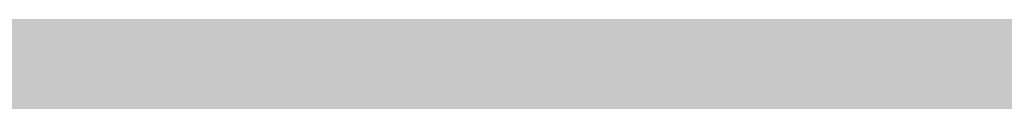
# Model space of a CAD drawing. Units: millimetres. Extents: x 0 to 2267, y 0 to 1823.
# Tile 51 of 256: x 1596.855 to 1600.369, y 1226.115 to 1226.386. Entities that reach past the tile are written whole.
import ezdxf

# ---------------------------------------------------------------- set-up
doc = ezdxf.new("R2010")
doc.units = ezdxf.units.MM
doc.header["$MEASUREMENT"] = 0
doc.layers.add('M-HATC', color=252, linetype='Continuous', lineweight=18)

msp = doc.modelspace()

# ---------------------------------------------------------------- hatches: boundary and pattern name
at = {"layer": 'M-HATC'}
h = msp.add_hatch(color=256, dxfattribs=at)
h.dxf.hatch_style = 1
h.paths.add_polyline_path([(2055.771, 1603.062), (1381.0868, 1603.062), (1381.0868, 1598.062), (2055.771, 1598.062)])
h.paths.add_polyline_path([(2055.771, 1598.062), (1381.0868, 1598.062), (1381.0868, 1593.062), (2055.771, 1593.062)])
h.paths.add_polyline_path([(2051.3074, 1536.7609), (1385.5504, 1536.7609), (1385.5504, 1526.7609), (1387.5504, 1526.7609), (1388.5366, 1525.0528), (1385.3319, 1521.2335), (1385.3319, 1521.2226), (2050.2542, 1522.7491), (2048.3212, 1525.0528), (2049.3074, 1526.7609), (2051.3074, 1526.7609)])
edge = h.paths.add_edge_path()
edge.add_arc((1847.5345, 1379.1492), 135, 222.603061, 222.890851, ccw=False)
edge.add_line((1748.1663, 1287.7656), (1683.0921, 1287.7656))
edge.add_arc((1583.7239, 1379.1492), 135, 317.109149, 317.396939, ccw=False)
edge.add_arc((1678.9686, 1290.6707), 5, 222.8909, 317.1091, ccw=False)
edge.add_arc((1774.2133, 1379.1492), 135, 222.603061, 222.890851, ccw=False)
edge.add_line((1674.8451, 1287.7656), (1609.7709, 1287.7656))
edge.add_arc((1510.4027, 1379.1492), 135, 317.109149, 317.396939, ccw=False)
edge.add_arc((1605.6474, 1290.6707), 5, 222.8909, 317.1091, ccw=False)
edge.add_arc((1700.8921, 1379.1492), 135, 222.603061, 222.890851, ccw=False)
edge.add_line((1601.5239, 1287.7656), (1536.4497, 1287.7656))
edge.add_arc((1437.0815, 1379.1492), 135, 317.109149, 317.396939, ccw=False)
edge.add_arc((1532.3262, 1290.6707), 5, 222.8909, 317.1091, ccw=False)
edge.add_arc((1627.5709, 1379.1492), 135, 222.603061, 222.890851, ccw=False)
edge.add_line((1528.2027, 1287.7656), (1505.9289, 1287.7656))
edge.add_spline(control_points=[(1505.9289, 1287.7656), (1504.2622, 1287.7656), (1504.2622, 1282.7656), (1505.9289, 1282.7656)], knot_values=[0, 0, 0, 0, 5, 5, 5, 5], degree=3, periodic=0)
edge.add_line((1505.9289, 1282.7656), (1930.9289, 1282.7656))
edge.add_spline(control_points=[(1930.9289, 1282.7656), (1932.5956, 1282.7656), (1932.5956, 1287.7656), (1930.9289, 1287.7656)], knot_values=[0, 0, 0, 0, 5, 5, 5, 5], degree=3, periodic=0)
edge.add_line((1930.9289, 1287.7656), (1903.0557, 1287.7656))
edge.add_arc((1803.6875, 1379.1492), 135, 317.109149, 317.396939, ccw=False)
edge.add_arc((1898.9322, 1290.6707), 5, 222.8909, 317.1091, ccw=False)
edge.add_arc((1994.1769, 1379.1492), 135, 222.603061, 222.890851, ccw=False)
edge.add_line((1894.8087, 1287.7656), (1829.7345, 1287.7656))
edge.add_arc((1730.3663, 1379.1492), 135, 317.109149, 317.396939, ccw=False)
edge.add_arc((1825.611, 1290.6707), 5, 222.8909, 317.1091, ccw=False)
edge.add_arc((1920.8557, 1379.1492), 135, 222.603061, 222.890851, ccw=False)
edge.add_line((1821.4875, 1287.7656), (1756.4133, 1287.7656))
edge.add_arc((1657.0451, 1379.1492), 135, 317.109149, 317.396939, ccw=False)
edge.add_arc((1752.2898, 1290.6707), 5, 222.8909, 317.1091, ccw=False)
edge = h.paths.add_edge_path()
edge.add_spline(control_points=[(1843.4289, 1227.2475), (1845.0956, 1227.2475), (1845.0956, 1232.2475), (1843.4289, 1232.2475)], knot_values=[0, 0, 0, 0, 5, 5, 5, 5], degree=3, periodic=0)
edge.add_line((1843.4289, 1232.2475), (1593.4289, 1232.2475))
edge.add_spline(control_points=[(1593.4289, 1232.2475), (1591.7622, 1232.2475), (1591.7622, 1227.2475), (1593.4289, 1227.2475)], knot_values=[0, 0, 0, 0, 5, 5, 5, 5], degree=3, periodic=0)
edge.add_line((1593.4289, 1227.2475), (1843.4289, 1227.2475))
h.paths.add_polyline_path([(1905.9289, 1127.4171), (1530.9289, 1127.4171, 0.414214), (1520.9289, 1117.4171), (1530.9289, 1117.4171), (1915.9289, 1117.4171, 0.414214)])
edge = h.paths.add_edge_path()
edge.add_arc((1397.0858, 1498.4078), 12.7299, 90.78215, 190.87871, ccw=False)
edge.add_line((1396.912, 1511.1365), (1428.0097, 1511.3488))
edge.add_line((1428.0097, 1511.3488), (1433.0097, 1511.3488))
edge.add_line((1433.0097, 1511.3488), (1434.439, 1511.3488))
edge.add_arc((1419.474, 1498.0804), 20, 41.561, 74.08211)
edge.add_line((1424.9592, 1517.3135), (1399.9351, 1517.2561))
edge.add_spline(control_points=[(1399.9307, 1517.2561), (1399.884, 1517.2131), (1399.8328, 1517.1689), (1399.7774, 1517.1236)], knot_values=[11.567499, 11.567499, 11.567499, 11.567499, 11.814249, 11.814249, 11.814249, 11.814249], degree=3, periodic=0)
edge.add_spline(control_points=[(1399.6328, 1517.0099), (1399.5831, 1516.9721), (1399.5307, 1516.9338), (1399.4759, 1516.8947)], knot_values=[11.167718, 11.167718, 11.167718, 11.167718, 11.365188, 11.365188, 11.365188, 11.365188], degree=3, periodic=0)
edge.add_spline(control_points=[(1399.3398, 1516.8001), (1399.1514, 1516.6719), (1398.9384, 1516.5377), (1398.704, 1516.3994)], knot_values=[10.376405, 10.376405, 10.376405, 10.376405, 11.00994, 11.00994, 11.00994, 11.00994], degree=3, periodic=0)
edge.add_spline(control_points=[(1398.6572, 1516.3719), (1398.5789, 1516.326), (1398.4983, 1516.2797), (1398.4155, 1516.2331)], knot_values=[10.125175, 10.125175, 10.125175, 10.125175, 10.334406, 10.334406, 10.334406, 10.334406], degree=3, periodic=0)
edge.add_spline(control_points=[(1398.2642, 1516.1487), (1398.196, 1516.1111), (1398.1263, 1516.0732), (1398.0555, 1516.0351)], knot_values=[9.832246, 9.832246, 9.832246, 9.832246, 9.999658, 9.999658, 9.999658, 9.999658], degree=3, periodic=0)
edge.add_spline(control_points=[(1397.9987, 1516.0048), (1397.7312, 1515.8621), (1397.446, 1515.7171), (1397.1466, 1515.5714)], knot_values=[9.161808, 9.161808, 9.161808, 9.161808, 9.787769, 9.787769, 9.787769, 9.787769], degree=3, periodic=0)
edge.add_spline(control_points=[(1397.1466, 1515.5714), (1396.8418, 1515.423), (1396.5222, 1515.274), (1396.1914, 1515.1262)], knot_values=[8.524455, 8.524455, 8.524455, 8.524455, 9.161808, 9.161808, 9.161808, 9.161808], degree=3, periodic=0)
edge.add_spline(control_points=[(1396.0777, 1515.0756), (1395.9854, 1515.0348), (1395.8922, 1514.994), (1395.7983, 1514.9534)], knot_values=[8.275193, 8.275193, 8.275193, 8.275193, 8.451726, 8.451726, 8.451726, 8.451726], degree=3, periodic=0)
edge.add_spline(control_points=[(1395.6018, 1514.8691), (1395.4997, 1514.8257), (1395.3968, 1514.7824), (1395.2932, 1514.7394)], knot_values=[7.962917, 7.962917, 7.962917, 7.962917, 8.152764, 8.152764, 8.152764, 8.152764], degree=3, periodic=0)
edge.add_spline(control_points=[(1395.2116, 1514.7057), (1394.8278, 1514.5475), (1394.4345, 1514.3929), (1394.0364, 1514.2442)], knot_values=[7.21254, 7.21254, 7.21254, 7.21254, 7.913148, 7.913148, 7.913148, 7.913148], degree=3, periodic=0)
edge.add_spline(control_points=[(1394.0364, 1514.2442), (1393.7076, 1514.1214), (1393.3754, 1514.0027), (1393.0427, 1513.8895)], knot_values=[6.633733, 6.633733, 6.633733, 6.633733, 7.21254, 7.21254, 7.21254, 7.21254], degree=3, periodic=0)
edge.add_spline(control_points=[(1392.8214, 1513.815), (1392.7198, 1513.7812), (1392.6181, 1513.7479), (1392.5166, 1513.7152)], knot_values=[6.328796, 6.328796, 6.328796, 6.328796, 6.505493, 6.505493, 6.505493, 6.505493], degree=3, periodic=0)
edge.add_spline(control_points=[(1392.5166, 1513.7152), (1392.3187, 1513.6515), (1392.1212, 1513.59), (1391.9244, 1513.531)], knot_values=[5.984605, 5.984605, 5.984605, 5.984605, 6.328796, 6.328796, 6.328796, 6.328796], degree=3, periodic=0)
edge.add_spline(control_points=[(1391.7915, 1513.4915), (1391.3122, 1513.3501), (1390.8384, 1513.2239), (1390.3784, 1513.1171)], knot_values=[5.066697, 5.066697, 5.066697, 5.066697, 5.907055, 5.907055, 5.907055, 5.907055], degree=3, periodic=0)
edge.add_spline(control_points=[(1390.3784, 1513.1171), (1390.1797, 1513.071), (1389.9836, 1513.0284), (1389.7907, 1512.9899)], knot_values=[4.70367, 4.70367, 4.70367, 4.70367, 5.066695, 5.066695, 5.066695, 5.066695], degree=3, periodic=0)
edge.add_spline(control_points=[(1389.422, 1512.9204), (1389.2459, 1512.8892), (1389.0729, 1512.8617), (1388.9036, 1512.8381)], knot_values=[4.130571, 4.130571, 4.130571, 4.130571, 4.469816, 4.469816, 4.469816, 4.469816], degree=3, periodic=0)
edge.add_spline(control_points=[(1388.9036, 1512.8381), (1388.591, 1512.7946), (1388.2911, 1512.7644), (1388.0071, 1512.7494)], knot_values=[3.504031, 3.504031, 3.504031, 3.504031, 4.130571, 4.130571, 4.130571, 4.130571], degree=3, periodic=0)
edge.add_spline(control_points=[(1387.9356, 1512.7459), (1387.8538, 1512.7423), (1387.7733, 1512.74), (1387.6944, 1512.739)], knot_values=[3.268866, 3.268866, 3.268866, 3.268866, 3.451164, 3.451164, 3.451164, 3.451164], degree=3, periodic=0)
edge.add_spline(control_points=[(1387.3351, 1512.7443), (1387.2076, 1512.7499), (1387.0847, 1512.7597), (1386.967, 1512.7739)], knot_values=[2.670686, 2.670686, 2.670686, 2.670686, 2.984, 2.984, 2.984, 2.984], degree=3, periodic=0)
edge.add_spline(control_points=[(1386.8327, 1512.7922), (1386.8209, 1512.7941), (1386.8092, 1512.7959), (1386.7975, 1512.7979)], knot_values=[2.516981, 2.516981, 2.516981, 2.516981, 2.549528, 2.549528, 2.549528, 2.549528], degree=3, periodic=0)
edge.add_spline(control_points=[(1386.4526, 1512.8735), (1386.4257, 1512.881), (1386.3993, 1512.889), (1386.3733, 1512.8972)], knot_values=[2.095869, 2.095869, 2.095869, 2.095869, 2.17941, 2.17941, 2.17941, 2.17941], degree=3, periodic=0)
edge.add_spline(control_points=[(1386.0691, 1513.0189), (1386.0634, 1513.0217), (1386.0577, 1513.0246), (1386.052, 1513.0275)], knot_values=[1.72453, 1.72453, 1.72453, 1.72453, 1.745933, 1.745933, 1.745933, 1.745933], degree=3, periodic=0)
edge.add_arc((1399.474, 1498.0804), 20, 131.82432, 180)
edge.add_arc((1630.3336, 1505.5484), 250.9708, 181.705176, 236.427975)
edge.add_arc((1605.3399, 1483.3044), 218.7822, 238.660829, 243.34961)
edge.add_arc((1647.0911, 1510.3592), 262.8986, 183.129836, 237.853442, ccw=False)
h.paths.add_polyline_path([(1406.5369, 1391.9644, 0.149382), (1491.5506, 1296.4418, -0.129517)], flags=17)
edge = h.paths.add_edge_path()
edge.add_arc((2037.3838, 1498.0804), 20, 0, 48.26587)
edge.add_spline(control_points=[(2050.6973, 1513.0052), (2050.6512, 1512.9847), (2050.6034, 1512.9655), (2050.5539, 1512.9477)], knot_values=[1.835652, 1.835652, 1.835652, 1.835652, 2.000781, 2.000781, 2.000781, 2.000781], degree=3, periodic=0)
edge.add_spline(control_points=[(2050.4616, 1512.9166), (2050.479, 1512.9221), (2050.4963, 1512.9277), (2050.5133, 1512.9335)], knot_values=[2.045477, 2.045477, 2.045477, 2.045477, 2.101389, 2.101389, 2.101389, 2.101389], degree=3, periodic=0)
edge.add_spline(control_points=[(2050.129, 1512.8342), (2050.1984, 1512.8473), (2050.2657, 1512.8623), (2050.3308, 1512.8792)], knot_values=[2.237629, 2.237629, 2.237629, 2.237629, 2.435841, 2.435841, 2.435841, 2.435841], degree=3, periodic=0)
edge.add_spline(control_points=[(2050.0946, 1512.8278), (2050.1061, 1512.8299), (2050.1176, 1512.832), (2050.129, 1512.8342)], knot_values=[2.435841, 2.435841, 2.435841, 2.435841, 2.468321, 2.468321, 2.468321, 2.468321], degree=3, periodic=0)
edge.add_spline(control_points=[(2049.7843, 1512.7851), (2049.8552, 1512.7922), (2049.9243, 1512.8008), (2049.9917, 1512.8109)], knot_values=[2.563852, 2.563852, 2.563852, 2.563852, 2.748541, 2.748541, 2.748541, 2.748541], degree=3, periodic=0)
edge.add_spline(control_points=[(2049.4052, 1512.7617), (2049.5364, 1512.7653), (2049.6629, 1512.773), (2049.7843, 1512.7851)], knot_values=[2.748541, 2.748541, 2.748541, 2.748541, 3.064882, 3.064882, 3.064882, 3.064882], degree=3, periodic=0)
edge.add_spline(control_points=[(2049.1698, 1512.7597), (2049.2336, 1512.7591), (2049.2965, 1512.7594), (2049.3584, 1512.7606)], knot_values=[3.102309, 3.102309, 3.102309, 3.102309, 3.2503, 3.2503, 3.2503, 3.2503], degree=3, periodic=0)
edge.add_spline(control_points=[(2048.8573, 1512.7691), (2048.9638, 1512.7638), (2049.068, 1512.7606), (2049.1698, 1512.7597)], knot_values=[3.2503, 3.2503, 3.2503, 3.2503, 3.486069, 3.486069, 3.486069, 3.486069], degree=3, periodic=0)
edge.add_spline(control_points=[(2048.6924, 1512.7789), (2048.3729, 1512.8009), (2048.0345, 1512.8411), (2047.6817, 1512.897)], knot_values=[3.606429, 3.606429, 3.606429, 3.606429, 4.2989, 4.2989, 4.2989, 4.2989], degree=3, periodic=0)
edge.add_spline(control_points=[(2047.6817, 1512.897), (2047.5458, 1512.9185), (2047.4077, 1512.9424), (2047.2678, 1512.9685)], knot_values=[4.2989, 4.2989, 4.2989, 4.2989, 4.565769, 4.565769, 4.565769, 4.565769], degree=3, periodic=0)
edge.add_spline(control_points=[(2047.2678, 1512.9685), (2047.1449, 1512.9914), (2047.0207, 1513.016), (2046.8951, 1513.0422)], knot_values=[4.565769, 4.565769, 4.565769, 4.565769, 4.799971, 4.799971, 4.799971, 4.799971], degree=3, periodic=0)
edge.add_spline(control_points=[(2046.8951, 1513.0422), (2046.5286, 1513.1188), (2046.1513, 1513.209), (2045.7676, 1513.3107)], knot_values=[4.799971, 4.799971, 4.799971, 4.799971, 5.483718, 5.483718, 5.483718, 5.483718], degree=3, periodic=0)
edge.add_spline(control_points=[(2045.7676, 1513.3107), (2045.3724, 1513.4154), (2044.9704, 1513.5322), (2044.5662, 1513.6588)], knot_values=[5.483718, 5.483718, 5.483718, 5.483718, 6.187866, 6.187866, 6.187866, 6.187866], degree=3, periodic=0)
edge.add_spline(control_points=[(2044.5662, 1513.6588), (2044.4149, 1513.7061), (2044.2633, 1513.7549), (2044.1116, 1513.8048)], knot_values=[6.187866, 6.187866, 6.187866, 6.187866, 6.451551, 6.451551, 6.451551, 6.451551], degree=3, periodic=0)
edge.add_spline(control_points=[(2044.1116, 1513.8048), (2043.9967, 1513.8427), (2043.8817, 1513.8813), (2043.7668, 1513.9205)], knot_values=[6.451551, 6.451551, 6.451551, 6.451551, 6.651434, 6.651434, 6.651434, 6.651434], degree=3, periodic=0)
edge.add_spline(control_points=[(2043.7668, 1513.9205), (2043.3716, 1514.0554), (2042.9774, 1514.1979), (2042.5886, 1514.3458)], knot_values=[6.651434, 6.651434, 6.651434, 6.651434, 7.338879, 7.338879, 7.338879, 7.338879], degree=3, periodic=0)
edge.add_spline(control_points=[(2042.5886, 1514.3458), (2042.1643, 1514.5071), (2041.7465, 1514.6749), (2041.3409, 1514.846)], knot_values=[7.338879, 7.338879, 7.338879, 7.338879, 8.089209, 8.089209, 8.089209, 8.089209], degree=3, periodic=0)
edge.add_spline(control_points=[(2041.3409, 1514.846), (2041.1028, 1514.9465), (2040.869, 1515.0481), (2040.6405, 1515.1502)], knot_values=[8.089209, 8.089209, 8.089209, 8.089209, 8.529587, 8.529587, 8.529587, 8.529587], degree=3, periodic=0)
edge.add_spline(control_points=[(2040.51, 1515.2089), (2040.0824, 1515.4022), (2039.6747, 1515.5971), (2039.295, 1515.7894)], knot_values=[8.613818, 8.613818, 8.613818, 8.613818, 9.44571, 9.44571, 9.44571, 9.44571], degree=3, periodic=0)
edge.add_spline(control_points=[(2039.295, 1515.7894), (2039.0618, 1515.9075), (2038.8391, 1516.0246), (2038.6288, 1516.1398)], knot_values=[9.44571, 9.44571, 9.44571, 9.44571, 9.956404, 9.956404, 9.956404, 9.956404], degree=3, periodic=0)
edge.add_spline(control_points=[(2038.6288, 1516.1398), (2038.5187, 1516.2001), (2038.4121, 1516.2598), (2038.309, 1516.3189)], knot_values=[9.956404, 9.956404, 9.956404, 9.956404, 10.223542, 10.223542, 10.223542, 10.223542], degree=3, periodic=0)
edge.add_spline(control_points=[(2038.309, 1516.3189), (2038.2138, 1516.3735), (2038.1216, 1516.4276), (2038.0328, 1516.481)], knot_values=[10.223542, 10.223542, 10.223542, 10.223542, 10.47051, 10.47051, 10.47051, 10.47051], degree=3, periodic=0)
edge.add_spline(control_points=[(2038.0328, 1516.481), (2037.7855, 1516.6296), (2037.5639, 1516.773), (2037.3722, 1516.909)], knot_values=[10.47051, 10.47051, 10.47051, 10.47051, 11.15767, 11.15767, 11.15767, 11.15767], degree=3, periodic=0)
edge.add_spline(control_points=[(2037.3722, 1516.909), (2037.2789, 1516.9752), (2037.1927, 1517.0396), (2037.1142, 1517.102)], knot_values=[11.15767, 11.15767, 11.15767, 11.15767, 11.49227, 11.49227, 11.49227, 11.49227], degree=3, periodic=0)
edge.add_spline(control_points=[(2036.8564, 1517.3259), (2036.9148, 1517.2692), (2036.9814, 1517.2103), (2037.0557, 1517.1492)], knot_values=[11.577341, 11.577341, 11.577341, 11.577341, 11.91035, 11.91035, 11.91035, 11.91035], degree=3, periodic=0)
edge.add_spline(control_points=[(2036.8074, 1517.3748), (2036.823, 1517.3587), (2036.8393, 1517.3424), (2036.8564, 1517.3259)], knot_values=[11.91035, 11.91035, 11.91035, 11.91035, 12.007402, 12.007402, 12.007402, 12.007402], degree=3, periodic=0)
edge.add_spline(control_points=[(2036.7017, 1517.494), (2036.7104, 1517.483), (2036.7196, 1517.4719), (2036.7291, 1517.4606)], knot_values=[12.184155, 12.184155, 12.184155, 12.184155, 12.255409, 12.255409, 12.255409, 12.255409], degree=3, periodic=0)
edge.add_spline(control_points=[(2036.6159, 1517.6205), (2036.62, 1517.613), (2036.6243, 1517.6055), (2036.6289, 1517.5979)], knot_values=[12.487913, 12.487913, 12.487913, 12.487913, 12.541035, 12.541035, 12.541035, 12.541035], degree=3, periodic=0)
edge.add_spline(control_points=[(2036.5635, 1517.786), (2036.5637, 1517.7794), (2036.5642, 1517.7726), (2036.565, 1517.7658)], knot_values=[12.911761, 12.911761, 12.911761, 12.911761, 12.968286, 12.968286, 12.968286, 12.968286], degree=3, periodic=0)
edge.add_spline(control_points=[(2036.6166, 1517.9304), (2036.6125, 1517.9259), (2036.6086, 1517.9212), (2036.6049, 1517.9165)], knot_values=[13.382527, 13.382527, 13.382527, 13.382527, 13.433791, 13.433791, 13.433791, 13.433791], degree=3, periodic=0)
edge.add_spline(control_points=[(2036.749, 1518.017), (2036.7361, 1518.0116), (2036.7239, 1518.006), (2036.7124, 1518.0002)], knot_values=[13.726299, 13.726299, 13.726299, 13.726299, 13.809928, 13.809928, 13.809928, 13.809928], degree=3, periodic=0)
edge.add_spline(control_points=[(2036.8604, 1518.0528), (2036.8386, 1518.0474), (2036.8181, 1518.0416), (2036.7988, 1518.0353)], knot_values=[13.910887, 13.910887, 13.910887, 13.910887, 14.02153, 14.02153, 14.02153, 14.02153], degree=3, periodic=0)
edge.add_line((2036.9639, 1518.0804), (2032.3838, 1518.0804))
edge.add_line((2032.3838, 1518.0804), (2027.3838, 1518.0804))
edge.add_line((2027.3838, 1518.0804), (2022.3838, 1518.0804))
edge.add_line((2022.3838, 1518.0804), (2017.3838, 1518.0804))
edge.add_arc((2017.3838, 1498.0804), 20, 90, 138.439)
edge.add_line((2002.4188, 1511.3488), (2003.8481, 1511.3488))
edge.add_line((2003.8481, 1511.3488), (2008.8481, 1511.3488))
edge.add_line((2008.8481, 1511.3488), (2039.772, 1511.1377))
edge.add_arc((2039.772, 1498.4078), 12.7299, -10.87871, 90, ccw=False)
edge.add_arc((1789.7668, 1510.3592), 262.8986, 302.146558, 356.870164, ccw=False)
edge.add_arc((1831.5179, 1483.3044), 218.7822, 296.65039, 301.339171)
edge.add_arc((1806.5242, 1505.5484), 250.9708, 303.572025, 358.294824)
h.paths.add_polyline_path([(2030.321, 1391.9644, -0.129517), (1945.3072, 1296.4418, 0.149382)], flags=17)
edge = h.paths.add_edge_path()
edge.add_spline(control_points=[(2037.2464, 1518.0821), (2037.2898, 1518.081), (2037.3355, 1518.0804), (2037.3838, 1518.0804)], knot_values=[0.000012, 0.000012, 0.000012, 0.000012, 0.144754, 0.144754, 0.144754, 0.144754], degree=3, periodic=0)
edge.add_line((2037.3357, 1518.0804), (2037.0096, 1518.0804))
edge.add_spline(control_points=[(2037.0096, 1518.0804), (2036.9822, 1518.0768), (2036.956, 1518.0727), (2036.9312, 1518.0681)], knot_values=[14.13465, 14.13465, 14.13465, 14.13465, 14.247197, 14.247197, 14.247197, 14.247197], degree=3, periodic=0)
edge.add_spline(control_points=[(2036.9312, 1518.0681), (2036.9276, 1518.0674), (2036.9241, 1518.0667), (2036.9205, 1518.0661)], knot_values=[14.118315, 14.118315, 14.118315, 14.118315, 14.13465, 14.13465, 14.13465, 14.13465], degree=3, periodic=0)
edge.add_spline(control_points=[(2036.9205, 1518.0661), (2036.9118, 1518.0644), (2036.9032, 1518.0626), (2036.8948, 1518.0608)], knot_values=[14.078086, 14.078086, 14.078086, 14.078086, 14.118315, 14.118315, 14.118315, 14.118315], degree=3, periodic=0)
edge.add_spline(control_points=[(2036.8948, 1518.0608), (2036.883, 1518.0583), (2036.8716, 1518.0556), (2036.8604, 1518.0528)], knot_values=[14.02153, 14.02153, 14.02153, 14.02153, 14.078086, 14.078086, 14.078086, 14.078086], degree=3, periodic=0)
edge.add_spline(control_points=[(2036.8604, 1518.0528), (2036.8386, 1518.0474), (2036.8181, 1518.0416), (2036.7988, 1518.0353)], knot_values=[13.910887, 13.910887, 13.910887, 13.910887, 14.02153, 14.02153, 14.02153, 14.02153], degree=3, periodic=0)
edge.add_spline(control_points=[(2036.7988, 1518.0353), (2036.7981, 1518.035), (2036.7974, 1518.0348), (2036.7967, 1518.0346)], knot_values=[13.906906, 13.906906, 13.906906, 13.906906, 13.910887, 13.910887, 13.910887, 13.910887], degree=3, periodic=0)
edge.add_spline(control_points=[(2036.7967, 1518.0346), (2036.7882, 1518.0318), (2036.7799, 1518.0289), (2036.7719, 1518.0259)], knot_values=[13.857826, 13.857826, 13.857826, 13.857826, 13.906906, 13.906906, 13.906906, 13.906906], degree=3, periodic=0)
edge.add_spline(control_points=[(2036.7719, 1518.0259), (2036.764, 1518.023), (2036.7564, 1518.02), (2036.749, 1518.017)], knot_values=[13.809928, 13.809928, 13.809928, 13.809928, 13.857826, 13.857826, 13.857826, 13.857826], degree=3, periodic=0)
edge.add_spline(control_points=[(2036.749, 1518.017), (2036.7361, 1518.0116), (2036.7239, 1518.006), (2036.7124, 1518.0002)], knot_values=[13.726299, 13.726299, 13.726299, 13.726299, 13.809928, 13.809928, 13.809928, 13.809928], degree=3, periodic=0)
edge.add_spline(control_points=[(2036.7124, 1518.0002), (2036.7121, 1518), (2036.7118, 1517.9999), (2036.7115, 1517.9997)], knot_values=[13.723993, 13.723993, 13.723993, 13.723993, 13.726299, 13.726299, 13.726299, 13.726299], degree=3, periodic=0)
edge.add_spline(control_points=[(2036.7115, 1517.9997), (2036.7063, 1517.9971), (2036.7013, 1517.9944), (2036.6965, 1517.9917)], knot_values=[13.686536, 13.686536, 13.686536, 13.686536, 13.723993, 13.723993, 13.723993, 13.723993], degree=3, periodic=0)
edge.add_spline(control_points=[(2036.6965, 1517.9917), (2036.6919, 1517.9891), (2036.6874, 1517.9865), (2036.6831, 1517.9839)], knot_values=[13.651251, 13.651251, 13.651251, 13.651251, 13.686536, 13.686536, 13.686536, 13.686536], degree=3, periodic=0)
edge.add_spline(control_points=[(2036.6831, 1517.9839), (2036.6764, 1517.9798), (2036.67, 1517.9757), (2036.6639, 1517.9714)], knot_values=[13.596804, 13.596804, 13.596804, 13.596804, 13.651251, 13.651251, 13.651251, 13.651251], degree=3, periodic=0)
edge.add_spline(control_points=[(2036.6639, 1517.9714), (2036.6636, 1517.9712), (2036.6633, 1517.9709), (2036.6629, 1517.9707)], knot_values=[13.593956, 13.593956, 13.593956, 13.593956, 13.596804, 13.596804, 13.596804, 13.596804], degree=3, periodic=0)
edge.add_spline(control_points=[(2036.6629, 1517.9707), (2036.6603, 1517.9689), (2036.6577, 1517.967), (2036.6552, 1517.9651)], knot_values=[13.570322, 13.570322, 13.570322, 13.570322, 13.593956, 13.593956, 13.593956, 13.593956], degree=3, periodic=0)
edge.add_spline(control_points=[(2036.6552, 1517.9651), (2036.6525, 1517.9631), (2036.6499, 1517.9611), (2036.6474, 1517.9591)], knot_values=[13.545477, 13.545477, 13.545477, 13.545477, 13.570322, 13.570322, 13.570322, 13.570322], degree=3, periodic=0)
edge.add_spline(control_points=[(2036.6474, 1517.9591), (2036.6472, 1517.9589), (2036.6471, 1517.9588), (2036.6469, 1517.9587)], knot_values=[13.543931, 13.543931, 13.543931, 13.543931, 13.545477, 13.545477, 13.545477, 13.545477], degree=3, periodic=0)
edge.add_spline(control_points=[(2036.6469, 1517.9587), (2036.6412, 1517.9541), (2036.6358, 1517.9494), (2036.6307, 1517.9447)], knot_values=[13.488237, 13.488237, 13.488237, 13.488237, 13.543931, 13.543931, 13.543931, 13.543931], degree=3, periodic=0)
edge.add_spline(control_points=[(2036.6307, 1517.9447), (2036.6282, 1517.9423), (2036.6257, 1517.9399), (2036.6233, 1517.9374)], knot_values=[13.460307, 13.460307, 13.460307, 13.460307, 13.488237, 13.488237, 13.488237, 13.488237], degree=3, periodic=0)
edge.add_spline(control_points=[(2036.6233, 1517.9374), (2036.6215, 1517.9356), (2036.6198, 1517.9338), (2036.6181, 1517.932)], knot_values=[13.439712, 13.439712, 13.439712, 13.439712, 13.460307, 13.460307, 13.460307, 13.460307], degree=3, periodic=0)
edge.add_spline(control_points=[(2036.6181, 1517.932), (2036.6176, 1517.9315), (2036.6171, 1517.9309), (2036.6166, 1517.9304)], knot_values=[13.433791, 13.433791, 13.433791, 13.433791, 13.439712, 13.439712, 13.439712, 13.439712], degree=3, periodic=0)
edge.add_spline(control_points=[(2036.6166, 1517.9304), (2036.6125, 1517.9259), (2036.6086, 1517.9212), (2036.6049, 1517.9165)], knot_values=[13.382527, 13.382527, 13.382527, 13.382527, 13.433791, 13.433791, 13.433791, 13.433791], degree=3, periodic=0)
edge.add_spline(control_points=[(2036.6049, 1517.9165), (2036.6026, 1517.9135), (2036.6004, 1517.9104), (2036.5982, 1517.9074)], knot_values=[13.350017, 13.350017, 13.350017, 13.350017, 13.382527, 13.382527, 13.382527, 13.382527], degree=3, periodic=0)
edge.add_spline(control_points=[(2036.5982, 1517.9074), (2036.5972, 1517.9059), (2036.5962, 1517.9043), (2036.5952, 1517.9028)], knot_values=[13.333922, 13.333922, 13.333922, 13.333922, 13.350017, 13.350017, 13.350017, 13.350017], degree=3, periodic=0)
edge.add_spline(control_points=[(2036.5952, 1517.9028), (2036.5945, 1517.9018), (2036.5939, 1517.9009), (2036.5933, 1517.8999)], knot_values=[13.323828, 13.323828, 13.323828, 13.323828, 13.333922, 13.333922, 13.333922, 13.333922], degree=3, periodic=0)
edge.add_spline(control_points=[(2036.5933, 1517.8999), (2036.5905, 1517.8955), (2036.5879, 1517.8909), (2036.5855, 1517.8864)], knot_values=[13.277545, 13.277545, 13.277545, 13.277545, 13.323828, 13.323828, 13.323828, 13.323828], degree=3, periodic=0)
edge.add_spline(control_points=[(2036.5855, 1517.8864), (2036.5836, 1517.8827), (2036.5817, 1517.8789), (2036.5801, 1517.8751)], knot_values=[13.240119, 13.240119, 13.240119, 13.240119, 13.277545, 13.277545, 13.277545, 13.277545], degree=3, periodic=0)
edge.add_spline(control_points=[(2036.5801, 1517.8751), (2036.5795, 1517.8739), (2036.579, 1517.8727), (2036.5785, 1517.8715)], knot_values=[13.228211, 13.228211, 13.228211, 13.228211, 13.240119, 13.240119, 13.240119, 13.240119], degree=3, periodic=0)
edge.add_spline(control_points=[(2036.5785, 1517.8715), (2036.578, 1517.8702), (2036.5774, 1517.869), (2036.5769, 1517.8677)], knot_values=[13.215717, 13.215717, 13.215717, 13.215717, 13.228211, 13.228211, 13.228211, 13.228211], degree=3, periodic=0)
edge.add_spline(control_points=[(2036.5769, 1517.8677), (2036.5755, 1517.864), (2036.5741, 1517.8603), (2036.5729, 1517.8565)], knot_values=[13.179847, 13.179847, 13.179847, 13.179847, 13.215717, 13.215717, 13.215717, 13.215717], degree=3, periodic=0)
edge.add_spline(control_points=[(2036.5729, 1517.8565), (2036.5713, 1517.8515), (2036.5699, 1517.8464), (2036.5687, 1517.8413)], knot_values=[13.132017, 13.132017, 13.132017, 13.132017, 13.179847, 13.179847, 13.179847, 13.179847], degree=3, periodic=0)
edge.add_spline(control_points=[(2036.5687, 1517.8413), (2036.5684, 1517.8402), (2036.5682, 1517.8392), (2036.568, 1517.8382)], knot_values=[13.122482, 13.122482, 13.122482, 13.122482, 13.132017, 13.132017, 13.132017, 13.132017], degree=3, periodic=0)
edge.add_spline(control_points=[(2036.568, 1517.8382), (2036.5676, 1517.8363), (2036.5672, 1517.8345), (2036.5669, 1517.8327)], knot_values=[13.105592, 13.105592, 13.105592, 13.105592, 13.122482, 13.122482, 13.122482, 13.122482], degree=3, periodic=0)
edge.add_spline(control_points=[(2036.5669, 1517.8327), (2036.5662, 1517.8292), (2036.5657, 1517.8257), (2036.5652, 1517.8222)], knot_values=[13.074063, 13.074063, 13.074063, 13.074063, 13.105592, 13.105592, 13.105592, 13.105592], degree=3, periodic=0)
edge.add_spline(control_points=[(2036.5652, 1517.8222), (2036.5652, 1517.8222), (2036.5652, 1517.8222), (2036.5652, 1517.8222)], knot_values=[13.074043, 13.074043, 13.074043, 13.074043, 13.074063, 13.074063, 13.074063, 13.074063], degree=3, periodic=0)
edge.add_spline(control_points=[(2036.5652, 1517.8222), (2036.5644, 1517.8164), (2036.5639, 1517.8106), (2036.5636, 1517.8046)], knot_values=[13.021884, 13.021884, 13.021884, 13.021884, 13.074043, 13.074043, 13.074043, 13.074043], degree=3, periodic=0)
edge.add_spline(control_points=[(2036.5636, 1517.8046), (2036.5636, 1517.804), (2036.5636, 1517.8034), (2036.5635, 1517.8028)], knot_values=[13.01674, 13.01674, 13.01674, 13.01674, 13.021884, 13.021884, 13.021884, 13.021884], degree=3, periodic=0)
edge.add_spline(control_points=[(2036.5635, 1517.8028), (2036.5634, 1517.8005), (2036.5634, 1517.7982), (2036.5634, 1517.7958)], knot_values=[12.996438, 12.996438, 12.996438, 12.996438, 13.01674, 13.01674, 13.01674, 13.01674], degree=3, periodic=0)
edge.add_spline(control_points=[(2036.5634, 1517.7958), (2036.5633, 1517.7926), (2036.5634, 1517.7893), (2036.5635, 1517.786)], knot_values=[12.968286, 12.968286, 12.968286, 12.968286, 12.996438, 12.996438, 12.996438, 12.996438], degree=3, periodic=0)
edge.add_spline(control_points=[(2036.5635, 1517.786), (2036.5637, 1517.7794), (2036.5642, 1517.7726), (2036.565, 1517.7658)], knot_values=[12.911761, 12.911761, 12.911761, 12.911761, 12.968286, 12.968286, 12.968286, 12.968286], degree=3, periodic=0)
edge.add_spline(control_points=[(2036.565, 1517.7658), (2036.565, 1517.7657), (2036.565, 1517.7656), (2036.565, 1517.7656)], knot_values=[12.911017, 12.911017, 12.911017, 12.911017, 12.911761, 12.911761, 12.911761, 12.911761], degree=3, periodic=0)
edge.add_spline(control_points=[(2036.565, 1517.7656), (2036.5654, 1517.7625), (2036.5658, 1517.7593), (2036.5663, 1517.7562)], knot_values=[12.88528, 12.88528, 12.88528, 12.88528, 12.911017, 12.911017, 12.911017, 12.911017], degree=3, periodic=0)
edge.add_spline(control_points=[(2036.5663, 1517.7562), (2036.5667, 1517.7534), (2036.5672, 1517.7506), (2036.5677, 1517.7478)], knot_values=[12.862519, 12.862519, 12.862519, 12.862519, 12.88528, 12.88528, 12.88528, 12.88528], degree=3, periodic=0)
edge.add_spline(control_points=[(2036.5677, 1517.7478), (2036.5678, 1517.7474), (2036.5679, 1517.7469), (2036.568, 1517.7465)], knot_values=[12.858885, 12.858885, 12.858885, 12.858885, 12.862519, 12.862519, 12.862519, 12.862519], degree=3, periodic=0)
edge.add_spline(control_points=[(2036.568, 1517.7465), (2036.5692, 1517.7399), (2036.5707, 1517.7332), (2036.5724, 1517.7264)], knot_values=[12.8053, 12.8053, 12.8053, 12.8053, 12.858885, 12.858885, 12.858885, 12.858885], degree=3, periodic=0)
edge.add_spline(control_points=[(2036.5724, 1517.7264), (2036.5734, 1517.7226), (2036.5745, 1517.7187), (2036.5756, 1517.7149)], knot_values=[12.775176, 12.775176, 12.775176, 12.775176, 12.8053, 12.8053, 12.8053, 12.8053], degree=3, periodic=0)
edge.add_spline(control_points=[(2036.5756, 1517.7149), (2036.5763, 1517.7125), (2036.577, 1517.7102), (2036.5778, 1517.7078)], knot_values=[12.756759, 12.756759, 12.756759, 12.756759, 12.775176, 12.775176, 12.775176, 12.775176], degree=3, periodic=0)
edge.add_spline(control_points=[(2036.5778, 1517.7078), (2036.5781, 1517.7067), (2036.5784, 1517.7057), (2036.5787, 1517.7047)], knot_values=[12.748742, 12.748742, 12.748742, 12.748742, 12.756759, 12.756759, 12.756759, 12.756759], degree=3, periodic=0)
edge.add_spline(control_points=[(2036.5787, 1517.7047), (2036.5808, 1517.6983), (2036.5831, 1517.6919), (2036.5856, 1517.6854)], knot_values=[12.69959, 12.69959, 12.69959, 12.69959, 12.748742, 12.748742, 12.748742, 12.748742], degree=3, periodic=0)
edge.add_spline(control_points=[(2036.5856, 1517.6854), (2036.5876, 1517.68), (2036.5898, 1517.6746), (2036.5921, 1517.6692)], knot_values=[12.659038, 12.659038, 12.659038, 12.659038, 12.69959, 12.69959, 12.69959, 12.69959], degree=3, periodic=0)
edge.add_spline(control_points=[(2036.5921, 1517.6692), (2036.594, 1517.6648), (2036.5959, 1517.6605), (2036.5979, 1517.6561)], knot_values=[12.626806, 12.626806, 12.626806, 12.626806, 12.659038, 12.659038, 12.659038, 12.659038], degree=3, periodic=0)
edge.add_spline(control_points=[(2036.5979, 1517.6561), (2036.5984, 1517.6551), (2036.5989, 1517.6541), (2036.5993, 1517.6531)], knot_values=[12.619394, 12.619394, 12.619394, 12.619394, 12.626806, 12.626806, 12.626806, 12.626806], degree=3, periodic=0)
edge.add_spline(control_points=[(2036.5993, 1517.6531), (2036.6043, 1517.6424), (2036.6099, 1517.6315), (2036.6159, 1517.6205)], knot_values=[12.541039, 12.541039, 12.541039, 12.541039, 12.619394, 12.619394, 12.619394, 12.619394], degree=3, periodic=0)
edge.add_spline(control_points=[(2036.6159, 1517.6205), (2036.6159, 1517.6205), (2036.6159, 1517.6205), (2036.6159, 1517.6205)], knot_values=[12.541035, 12.541035, 12.541035, 12.541035, 12.541039, 12.541039, 12.541039, 12.541039], degree=3, periodic=0)
edge.add_spline(control_points=[(2036.6159, 1517.6205), (2036.62, 1517.613), (2036.6243, 1517.6055), (2036.6289, 1517.5979)], knot_values=[12.487913, 12.487913, 12.487913, 12.487913, 12.541035, 12.541035, 12.541035, 12.541035], degree=3, periodic=0)
edge.add_spline(control_points=[(2036.6289, 1517.5979), (2036.6326, 1517.5916), (2036.6365, 1517.5853), (2036.6406, 1517.5789)], knot_values=[12.443982, 12.443982, 12.443982, 12.443982, 12.487913, 12.487913, 12.487913, 12.487913], degree=3, periodic=0)
edge.add_spline(control_points=[(2036.6406, 1517.5789), (2036.6414, 1517.5776), (2036.6423, 1517.5763), (2036.6431, 1517.5749)], knot_values=[12.434996, 12.434996, 12.434996, 12.434996, 12.443982, 12.443982, 12.443982, 12.443982], degree=3, periodic=0)
edge.add_spline(control_points=[(2036.6431, 1517.5749), (2036.6531, 1517.5596), (2036.6639, 1517.5439), (2036.6756, 1517.528)], knot_values=[12.329647, 12.329647, 12.329647, 12.329647, 12.434996, 12.434996, 12.434996, 12.434996], degree=3, periodic=0)
edge.add_spline(control_points=[(2036.6756, 1517.528), (2036.6839, 1517.5168), (2036.6925, 1517.5055), (2036.7017, 1517.494)], knot_values=[12.255409, 12.255409, 12.255409, 12.255409, 12.329647, 12.329647, 12.329647, 12.329647], degree=3, periodic=0)
edge.add_spline(control_points=[(2036.7017, 1517.494), (2036.7104, 1517.483), (2036.7196, 1517.4719), (2036.7291, 1517.4606)], knot_values=[12.184155, 12.184155, 12.184155, 12.184155, 12.255409, 12.255409, 12.255409, 12.255409], degree=3, periodic=0)
edge.add_spline(control_points=[(2036.7291, 1517.4606), (2036.7436, 1517.4435), (2036.759, 1517.4262), (2036.7753, 1517.4085)], knot_values=[12.075961, 12.075961, 12.075961, 12.075961, 12.184155, 12.184155, 12.184155, 12.184155], degree=3, periodic=0)
edge.add_spline(control_points=[(2036.7753, 1517.4085), (2036.7763, 1517.4075), (2036.7773, 1517.4064), (2036.7783, 1517.4054)], knot_values=[12.069502, 12.069502, 12.069502, 12.069502, 12.075961, 12.075961, 12.075961, 12.075961], degree=3, periodic=0)
edge.add_spline(control_points=[(2036.7783, 1517.4054), (2036.7877, 1517.3953), (2036.7974, 1517.385), (2036.8074, 1517.3748)], knot_values=[12.007402, 12.007402, 12.007402, 12.007402, 12.069502, 12.069502, 12.069502, 12.069502], degree=3, periodic=0)
edge.add_spline(control_points=[(2036.8074, 1517.3748), (2036.823, 1517.3587), (2036.8393, 1517.3424), (2036.8564, 1517.3259)], knot_values=[11.91035, 11.91035, 11.91035, 11.91035, 12.007402, 12.007402, 12.007402, 12.007402], degree=3, periodic=0)
edge.add_spline(control_points=[(2036.8564, 1517.3259), (2036.9148, 1517.2692), (2036.9814, 1517.2103), (2037.0557, 1517.1492)], knot_values=[11.577341, 11.577341, 11.577341, 11.577341, 11.91035, 11.91035, 11.91035, 11.91035], degree=3, periodic=0)
edge.add_spline(control_points=[(2037.0557, 1517.1492), (2037.0747, 1517.1336), (2037.0942, 1517.1179), (2037.1142, 1517.102)], knot_values=[11.49227, 11.49227, 11.49227, 11.49227, 11.577341, 11.577341, 11.577341, 11.577341], degree=3, periodic=0)
edge.add_spline(control_points=[(2037.1142, 1517.102), (2037.1927, 1517.0396), (2037.2789, 1516.9752), (2037.3722, 1516.909)], knot_values=[11.15767, 11.15767, 11.15767, 11.15767, 11.49227, 11.49227, 11.49227, 11.49227], degree=3, periodic=0)
edge.add_spline(control_points=[(2037.3722, 1516.909), (2037.5639, 1516.773), (2037.7855, 1516.6296), (2038.0328, 1516.481)], knot_values=[10.47051, 10.47051, 10.47051, 10.47051, 11.15767, 11.15767, 11.15767, 11.15767], degree=3, periodic=0)
edge.add_spline(control_points=[(2038.0328, 1516.481), (2038.1216, 1516.4276), (2038.2138, 1516.3735), (2038.309, 1516.3189)], knot_values=[10.223542, 10.223542, 10.223542, 10.223542, 10.47051, 10.47051, 10.47051, 10.47051], degree=3, periodic=0)
edge.add_spline(control_points=[(2038.309, 1516.3189), (2038.4121, 1516.2598), (2038.5187, 1516.2001), (2038.6288, 1516.1398)], knot_values=[9.956404, 9.956404, 9.956404, 9.956404, 10.223542, 10.223542, 10.223542, 10.223542], degree=3, periodic=0)
edge.add_spline(control_points=[(2038.6288, 1516.1398), (2038.8391, 1516.0246), (2039.0618, 1515.9075), (2039.295, 1515.7894)], knot_values=[9.44571, 9.44571, 9.44571, 9.44571, 9.956404, 9.956404, 9.956404, 9.956404], degree=3, periodic=0)
edge.add_spline(control_points=[(2039.295, 1515.7894), (2039.6747, 1515.5971), (2040.0824, 1515.4022), (2040.51, 1515.2089)], knot_values=[8.613818, 8.613818, 8.613818, 8.613818, 9.44571, 9.44571, 9.44571, 9.44571], degree=3, periodic=0)
edge.add_spline(control_points=[(2040.51, 1515.2089), (2040.5533, 1515.1893), (2040.5968, 1515.1697), (2040.6405, 1515.1502)], knot_values=[8.529587, 8.529587, 8.529587, 8.529587, 8.613818, 8.613818, 8.613818, 8.613818], degree=3, periodic=0)
edge.add_spline(control_points=[(2040.6405, 1515.1502), (2040.869, 1515.0481), (2041.1028, 1514.9465), (2041.3409, 1514.846)], knot_values=[8.089209, 8.089209, 8.089209, 8.089209, 8.529587, 8.529587, 8.529587, 8.529587], degree=3, periodic=0)
edge.add_spline(control_points=[(2041.3409, 1514.846), (2041.7465, 1514.6749), (2042.1643, 1514.5071), (2042.5886, 1514.3458)], knot_values=[7.338879, 7.338879, 7.338879, 7.338879, 8.089209, 8.089209, 8.089209, 8.089209], degree=3, periodic=0)
edge.add_spline(control_points=[(2042.5886, 1514.3458), (2042.9774, 1514.1979), (2043.3716, 1514.0554), (2043.7668, 1513.9205)], knot_values=[6.651434, 6.651434, 6.651434, 6.651434, 7.338879, 7.338879, 7.338879, 7.338879], degree=3, periodic=0)
edge.add_spline(control_points=[(2043.7668, 1513.9205), (2043.8817, 1513.8813), (2043.9967, 1513.8427), (2044.1116, 1513.8048)], knot_values=[6.451551, 6.451551, 6.451551, 6.451551, 6.651434, 6.651434, 6.651434, 6.651434], degree=3, periodic=0)
edge.add_spline(control_points=[(2044.1116, 1513.8048), (2044.2633, 1513.7549), (2044.4149, 1513.7061), (2044.5662, 1513.6588)], knot_values=[6.187866, 6.187866, 6.187866, 6.187866, 6.451551, 6.451551, 6.451551, 6.451551], degree=3, periodic=0)
edge.add_spline(control_points=[(2044.5662, 1513.6588), (2044.9704, 1513.5322), (2045.3724, 1513.4154), (2045.7676, 1513.3107)], knot_values=[5.483718, 5.483718, 5.483718, 5.483718, 6.187866, 6.187866, 6.187866, 6.187866], degree=3, periodic=0)
edge.add_spline(control_points=[(2045.7676, 1513.3107), (2046.1513, 1513.209), (2046.5286, 1513.1188), (2046.8951, 1513.0422)], knot_values=[4.799971, 4.799971, 4.799971, 4.799971, 5.483718, 5.483718, 5.483718, 5.483718], degree=3, periodic=0)
edge.add_spline(control_points=[(2046.8951, 1513.0422), (2047.0207, 1513.016), (2047.1449, 1512.9914), (2047.2678, 1512.9685)], knot_values=[4.565769, 4.565769, 4.565769, 4.565769, 4.799971, 4.799971, 4.799971, 4.799971], degree=3, periodic=0)
edge.add_spline(control_points=[(2047.2678, 1512.9685), (2047.4077, 1512.9424), (2047.5458, 1512.9185), (2047.6817, 1512.897)], knot_values=[4.2989, 4.2989, 4.2989, 4.2989, 4.565769, 4.565769, 4.565769, 4.565769], degree=3, periodic=0)
edge.add_spline(control_points=[(2047.6817, 1512.897), (2048.0345, 1512.8411), (2048.3729, 1512.8009), (2048.6924, 1512.7789)], knot_values=[3.606429, 3.606429, 3.606429, 3.606429, 4.2989, 4.2989, 4.2989, 4.2989], degree=3, periodic=0)
edge.add_spline(control_points=[(2048.6924, 1512.7789), (2048.7479, 1512.7751), (2048.8029, 1512.7718), (2048.8573, 1512.7691)], knot_values=[3.486069, 3.486069, 3.486069, 3.486069, 3.606429, 3.606429, 3.606429, 3.606429], degree=3, periodic=0)
edge.add_spline(control_points=[(2048.8573, 1512.7691), (2048.9638, 1512.7638), (2049.068, 1512.7606), (2049.1698, 1512.7597)], knot_values=[3.2503, 3.2503, 3.2503, 3.2503, 3.486069, 3.486069, 3.486069, 3.486069], degree=3, periodic=0)
edge.add_spline(control_points=[(2049.1698, 1512.7597), (2049.2336, 1512.7591), (2049.2965, 1512.7594), (2049.3584, 1512.7606)], knot_values=[3.102309, 3.102309, 3.102309, 3.102309, 3.2503, 3.2503, 3.2503, 3.2503], degree=3, periodic=0)
edge.add_spline(control_points=[(2049.3584, 1512.7606), (2049.3741, 1512.7609), (2049.3897, 1512.7613), (2049.4052, 1512.7617)], knot_values=[3.064882, 3.064882, 3.064882, 3.064882, 3.102309, 3.102309, 3.102309, 3.102309], degree=3, periodic=0)
edge.add_spline(control_points=[(2049.4052, 1512.7617), (2049.5364, 1512.7653), (2049.6629, 1512.773), (2049.7843, 1512.7851)], knot_values=[2.748541, 2.748541, 2.748541, 2.748541, 3.064882, 3.064882, 3.064882, 3.064882], degree=3, periodic=0)
edge.add_spline(control_points=[(2049.7843, 1512.7851), (2049.8552, 1512.7922), (2049.9243, 1512.8008), (2049.9917, 1512.8109)], knot_values=[2.563852, 2.563852, 2.563852, 2.563852, 2.748541, 2.748541, 2.748541, 2.748541], degree=3, periodic=0)
edge.add_spline(control_points=[(2049.9917, 1512.8109), (2050.0265, 1512.8161), (2050.0608, 1512.8218), (2050.0946, 1512.8278)], knot_values=[2.468321, 2.468321, 2.468321, 2.468321, 2.563852, 2.563852, 2.563852, 2.563852], degree=3, periodic=0)
edge.add_spline(control_points=[(2050.0946, 1512.8278), (2050.1061, 1512.8299), (2050.1176, 1512.832), (2050.129, 1512.8342)], knot_values=[2.435841, 2.435841, 2.435841, 2.435841, 2.468321, 2.468321, 2.468321, 2.468321], degree=3, periodic=0)
edge.add_spline(control_points=[(2050.129, 1512.8342), (2050.1984, 1512.8473), (2050.2657, 1512.8623), (2050.3308, 1512.8792)], knot_values=[2.237629, 2.237629, 2.237629, 2.237629, 2.435841, 2.435841, 2.435841, 2.435841], degree=3, periodic=0)
edge.add_spline(control_points=[(2050.3308, 1512.8792), (2050.3754, 1512.8908), (2050.4191, 1512.9032), (2050.4616, 1512.9166)], knot_values=[2.101389, 2.101389, 2.101389, 2.101389, 2.237629, 2.237629, 2.237629, 2.237629], degree=3, periodic=0)
edge.add_spline(control_points=[(2050.4616, 1512.9166), (2050.479, 1512.9221), (2050.4963, 1512.9277), (2050.5133, 1512.9335)], knot_values=[2.045477, 2.045477, 2.045477, 2.045477, 2.101389, 2.101389, 2.101389, 2.101389], degree=3, periodic=0)
edge.add_spline(control_points=[(2050.5133, 1512.9335), (2050.527, 1512.9382), (2050.5405, 1512.9429), (2050.5539, 1512.9477)], knot_values=[2.000781, 2.000781, 2.000781, 2.000781, 2.045477, 2.045477, 2.045477, 2.045477], degree=3, periodic=0)
edge.add_spline(control_points=[(2050.5539, 1512.9477), (2050.6034, 1512.9655), (2050.6512, 1512.9847), (2050.6973, 1513.0052)], knot_values=[1.835652, 1.835652, 1.835652, 1.835652, 2.000781, 2.000781, 2.000781, 2.000781], degree=3, periodic=0)
edge.add_arc((2037.3838, 1498.0804), 20, 48.26587, 90.12993)
edge = h.paths.add_edge_path(flags=16)
edge.add_spline(control_points=[(1386.1389, 1512.9859), (1388.92, 1511.7395), (1398.0387, 1515.5187), (1399.9307, 1517.2561)], knot_values=[1.831046, 1.831046, 1.831046, 1.831046, 11.814249, 11.814249, 11.814249, 11.814249], degree=3, periodic=0)
edge.add_line((1399.9307, 1517.2561), (1393.7435, 1517.2419))
edge.add_arc((1399.474, 1498.0804), 20, 106.6501, 131.8173)
h = msp.add_hatch(color=256, dxfattribs=at)
h.dxf.hatch_style = 1
h.paths.add_polyline_path([(2042.8886, 1580.1796), (2055.771, 1593.062), (1381.0868, 1593.062), (1393.9692, 1580.1796), (1374.086, 1560.2964), (2062.7718, 1560.2964)])
h.paths.add_polyline_path([(1843.4289, 1201.3297), (1843.4289, 1227.2475), (1593.4289, 1227.2475), (1593.4289, 1201.3297, -0.228274), (1574.5989, 1162.2346), (1530.9289, 1127.4171), (1905.9289, 1127.4171), (1862.2589, 1162.2346, -0.228274)])

doc.saveas('drawing.dxf')
